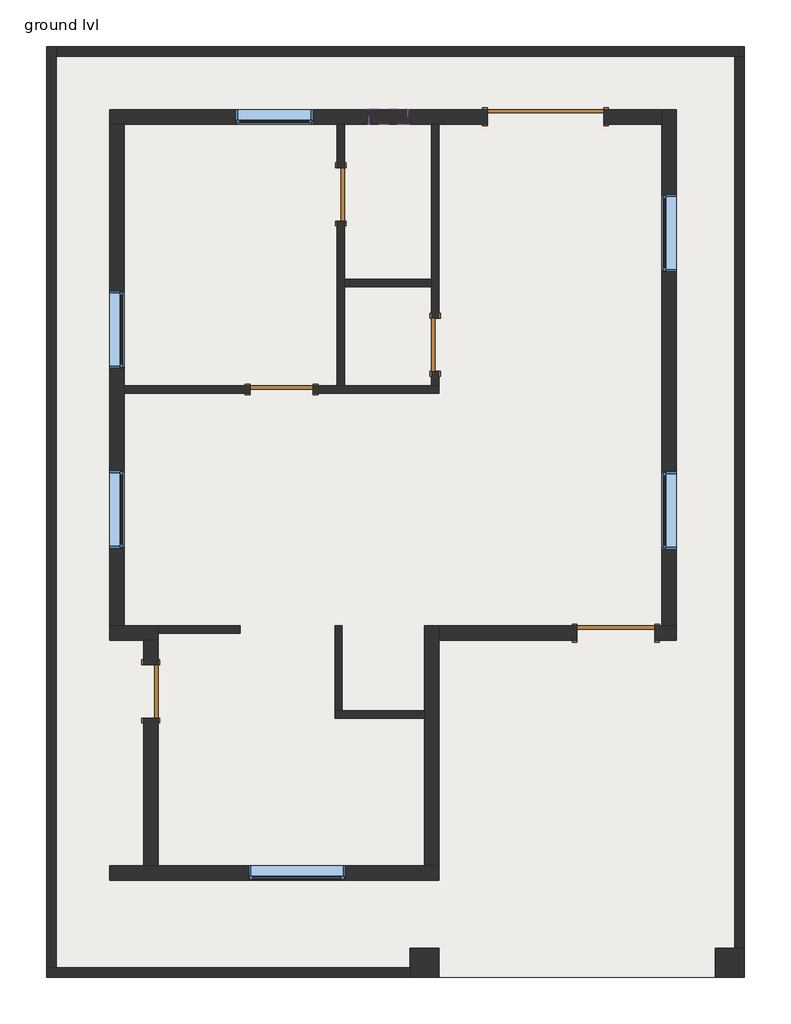
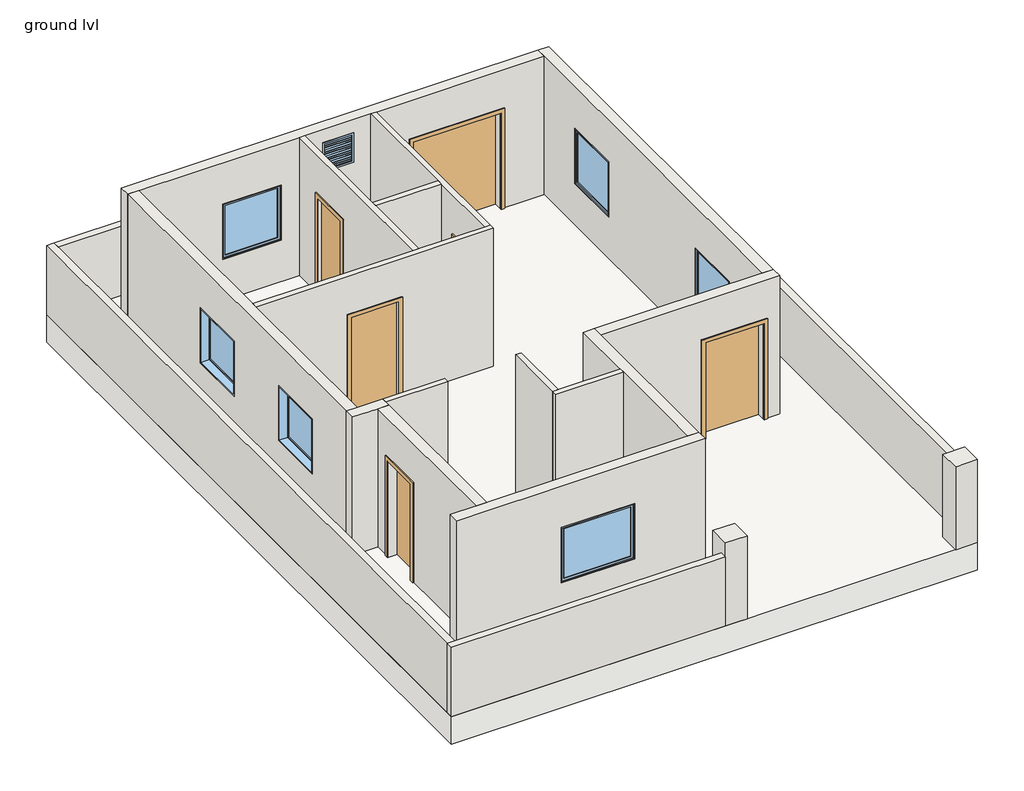
# One storey: 21 walls, 7 windows, 6 doors, 1 slab.
"""IFC4 building model written with IfcOpenShell, lengths in millimetres."""

from ifc_helpers import new_model, si_unit, frame, origin, origin_with_axes, place, context, project, spatial, polyline, outline, extrude, faceted_brep, transform, mapped, element, save
from components import single_flush_6_d_bd5e0b13, single_flush_d1_2531c3a3, single_flush_d2_53d9c022, single_flush_d3_0217d254, single_flush_d4_f1814d11, single_flush_d2_19300210, fixed_4_2_76f305d9, fixed_5_145d3b12, window_louvers_2_f2d8fef0

model = new_model("IFC4")

# Units and contexts
model_context = context("Model", 3, world=origin())
ifc_project = project(units=[si_unit("LENGTHUNIT", "METRE", prefix="MILLI")], contexts=[model_context])

# Site, building, storey
site = spatial("IfcSite", under=ifc_project)
building = spatial("IfcBuilding", under=site)
storey = spatial("IfcBuildingStorey", under=building, Name="ground lvl", Elevation=0.0)

# Doors
placement = place(None, origin())
single_flush_6_d_shape = single_flush_6_d_bd5e0b13(model_context)
element("IfcDoor", 1, ObjectType="Single-Flush : 6' d", at=placement, inside=storey, context=model_context, shape_type="MappedRepresentation", body=[
    mapped(single_flush_6_d_shape, transform((-16061.6899593, 8004.4908098, 0.0), x_axis=(1.0, 0.0, 0.0), y_axis=(0.0, 1.0, 0.0), z_axis=(0.0, 0.0, 1.0))),
])
single_flush_d1_shape = single_flush_d1_2531c3a3(model_context)
element("IfcDoor", 2, ObjectType="Single-Flush : d1", at=placement, inside=storey, context=model_context, shape_type="MappedRepresentation", body=[
    mapped(single_flush_d1_shape, transform((-14956.7899593, -110.8091902, 0.0), x_axis=(1.0, 0.0, 0.0), y_axis=(0.0, 1.0, 0.0), z_axis=(0.0, 0.0, 1.0))),
])
single_flush_d2_shape = single_flush_d2_53d9c022(model_context)
element("IfcDoor", 3, ObjectType="Single-Flush : d2", at=placement, inside=storey, context=model_context, shape_type="MappedRepresentation", body=[
    mapped(single_flush_d2_shape, transform((-22271.9899593, -1025.2091902, 0.0), x_axis=(0.0, 1.0, 0.0), y_axis=(-1.0, 0.0, 0.0), z_axis=(0.0, 0.0, 1.0))),
])
single_flush_d3_shape = single_flush_d3_0217d254(model_context)
element("IfcDoor", 4, ObjectType="Single-Flush : d3", at=placement, inside=storey, context=model_context, shape_type="MappedRepresentation", body=[
    mapped(single_flush_d3_shape, transform((-20214.5899593, 3718.2408098, 0.0), x_axis=(1.0, 0.0, 0.0), y_axis=(0.0, 1.0, 0.0), z_axis=(0.0, 0.0, 1.0))),
])
single_flush_d4_shape = single_flush_d4_f1814d11(model_context)
element("IfcDoor", 5, ObjectType="Single-Flush : d4", at=placement, inside=storey, context=model_context, shape_type="MappedRepresentation", body=[
    mapped(single_flush_d4_shape, transform((-19281.1399593, 6785.2908098, 0.0), x_axis=(0.0, -1.0, 0.0), y_axis=(1.0, 0.0, 0.0), z_axis=(0.0, 0.0, 1.0))),
])
single_flush_d2_2_shape = single_flush_d2_19300210(model_context)
element("IfcDoor", 6, ObjectType="Single-Flush : d4", at=placement, inside=storey, context=model_context, shape_type="MappedRepresentation", body=[
    mapped(single_flush_d2_2_shape, transform((-17795.2399593, 4423.0908098, 0.0), x_axis=(0.0, -1.0, 0.0), y_axis=(1.0, 0.0, 0.0), z_axis=(0.0, 0.0, 1.0))),
])

# Slab
element("IfcSlab", 7, ObjectType="2'", at=placement, inside=storey, context=model_context, shape_type="SweptSolid", body=[
    extrude(outline(polyline([(-23910.2899593, 9109.3908098), (-12937.4899593, 9109.3908098), (-12937.4899593, -5521.0091902), (-23910.2899593, -5521.0091902), (-23910.2899593, 9109.3908098)])), frame((0.0, 0.0, -609.6), z_axis=(0.0, 0.0, 1.0), x_axis=(1.0, 0.0, 0.0)), (0.0, 0.0, 1.0), 609.6),
])

# Walls
element("IfcWall", 8, ObjectType="1'6\" w", at=placement, inside=storey, context=model_context, shape_type="Brep", body=[
    faceted_brep([(-18195.2899593, -5521.0091902, 0.0), (-17738.0899593, -5521.0091902, 0.0), (-17738.0899593, -5521.0091902, 1828.8), (-18195.2899593, -5521.0091902, 1828.8), (-18195.2899593, -5521.0091902, 1524.0), (-18195.2899593, -5063.8091902, 0.0), (-18195.2899593, -5063.8091902, 1828.8), (-17738.0899593, -5063.8091902, 1828.8), (-17738.0899593, -5063.8091902, 0.0), (-18195.2899593, -5368.6091902, 0.0)], [[[0, 1, 2, 3, 4]], [[5, 6, 7, 8]], [[1, 0, 9, 5, 8]], [[2, 1, 8, 7]], [[3, 2, 7, 6]], [[0, 4, 3, 6, 5, 9]]]),
])
element("IfcWall", 9, ObjectType="1'6\" w", at=placement, inside=storey, context=model_context, shape_type="Brep", body=[
    faceted_brep([(-13394.6899593, -5521.0091902, 0.0), (-12937.4899593, -5521.0091902, 0.0), (-12937.4899593, -5521.0091902, 1828.8), (-13394.6899593, -5521.0091902, 1828.8), (-13394.6899593, -5063.8091902, 0.0), (-13394.6899593, -5063.8091902, 1828.8), (-12937.4899593, -5063.8091902, 1828.8), (-12937.4899593, -5063.8091902, 1524.0), (-12937.4899593, -5063.8091902, 0.0), (-13089.8899593, -5063.8091902, 0.0)], [[[0, 1, 2, 3]], [[4, 5, 6, 7, 8, 9]], [[1, 0, 4, 9, 8]], [[3, 2, 6, 5]], [[0, 3, 5, 4]], [[2, 1, 8, 7, 6]]]),
])
element("IfcWall", 10, ObjectType="4.5\" w", at=placement, inside=storey, context=model_context, shape_type="SweptSolid", body=[
    extrude(outline(polyline([(-20862.2899593, -110.8091902), (-22157.6899593, -110.8091902), (-22157.6899593, 3.4908098), (-20862.2899593, 3.4908098), (-20862.2899593, -110.8091902)])), origin_with_axes(), (0.0, 0.0, 1.0), 3048.0),
])
element("IfcWall", 11, ObjectType="4.5\" w", at=placement, inside=storey, context=model_context, shape_type="Brep", body=[
    faceted_brep([(-17966.6899593, -1330.0091901, 0.0), (-19262.0899593, -1330.0091901, 0.0), (-19376.3899593, -1330.0091901, 0.0), (-19376.3899593, -1330.0091901, 3048.0), (-19262.0899593, -1330.0091901, 3048.0), (-17966.6899593, -1330.0091901, 3048.0), (-17966.6899593, -1444.3091901, 0.0), (-17966.6899593, -1444.3091901, 3048.0), (-19376.3899593, -1444.3091901, 3048.0), (-19376.3899593, -1444.3091901, 0.0)], [[[0, 1, 2, 3, 4, 5]], [[6, 7, 8, 9]], [[2, 1, 0, 6, 9]], [[5, 4, 3, 8, 7]], [[0, 5, 7, 6]], [[3, 2, 9, 8]]]),
])
element("IfcWall", 12, ObjectType="4.5\" w", at=placement, inside=storey, context=model_context, shape_type="SweptSolid", body=[
    extrude(outline(polyline([(-19262.0899593, 3.4908098), (-19262.0899593, -1330.0091901), (-19376.3899593, -1330.0091901), (-19376.3899593, 3.4908098), (-19262.0899593, 3.4908098)])), origin_with_axes(), (0.0, 0.0, 1.0), 3048.0),
])
element("IfcWall", 13, ObjectType="4.5\" w", at=placement, inside=storey, context=model_context, shape_type="Brep", body=[
    faceted_brep([(-19719.2899593, 3661.0908098, 2133.6), (-19719.2899593, 3661.0908098, 0.0), (-17738.0899593, 3661.0908098, 0.0), (-17738.0899593, 3661.0908098, 3048.0), (-22691.0899593, 3661.0908098, 3048.0), (-22691.0899593, 3661.0908098, 0.0), (-20709.8899593, 3661.0908098, 0.0), (-20709.8899593, 3661.0908098, 2133.6), (-17738.0899593, 3775.3908098, 0.0), (-17852.3899593, 3775.3908098, 0.0), (-19223.9899593, 3775.3908098, 0.0), (-19338.2899593, 3775.3908098, 0.0), (-19719.2899593, 3775.3908098, 0.0), (-19719.2899593, 3775.3908098, 2133.6), (-20709.8899593, 3775.3908098, 2133.6), (-20709.8899593, 3775.3908098, 0.0), (-22691.0899593, 3775.3908098, 0.0), (-22691.0899593, 3775.3908098, 3048.0), (-19338.2899593, 3775.3908098, 3048.0), (-19223.9899593, 3775.3908098, 3048.0), (-17852.3899593, 3775.3908098, 3048.0), (-17738.0899593, 3775.3908098, 3048.0)], [[[0, 1, 2, 3, 4, 5, 6, 7]], [[8, 9, 10, 11, 12, 13, 14, 15, 16, 17, 18, 19, 20, 21]], [[6, 5, 16, 15]], [[2, 1, 12, 11, 10, 9, 8]], [[4, 3, 21, 20, 19, 18, 17]], [[5, 4, 17, 16]], [[3, 2, 8, 21]], [[13, 12, 1, 0]], [[14, 13, 0, 7]], [[15, 14, 7, 6]]]),
])
element("IfcWall", 14, ObjectType="4.5\" w", at=placement, inside=storey, context=model_context, shape_type="Brep", body=[
    faceted_brep([(-17738.0899593, 3775.3908098, 0.0), (-17738.0899593, 4003.9908098, 0.0), (-17738.0899593, 4003.9908098, 2133.6), (-17738.0899593, 4842.1908098, 2133.6), (-17738.0899593, 4842.1908098, 0.0), (-17738.0899593, 7890.1908098, 0.0), (-17738.0899593, 7890.1908098, 3048.0), (-17738.0899593, 3775.3908098, 3048.0), (-17852.3899593, 4003.9908098, 2133.6), (-17852.3899593, 4003.9908098, 0.0), (-17852.3899593, 3775.3908098, 0.0), (-17852.3899593, 3775.3908098, 3048.0), (-17852.3899593, 5337.4908098, 3048.0), (-17852.3899593, 5451.7908098, 3048.0), (-17852.3899593, 7890.1908098, 3048.0), (-17852.3899593, 7890.1908098, 0.0), (-17852.3899593, 5451.7908098, 0.0), (-17852.3899593, 5337.4908098, 0.0), (-17852.3899593, 4842.1908098, 0.0), (-17852.3899593, 4842.1908098, 2133.6)], [[[0, 1, 2, 3, 4, 5, 6, 7]], [[8, 9, 10, 11, 12, 13, 14, 15, 16, 17, 18, 19]], [[10, 9, 1, 0]], [[18, 17, 16, 15, 5, 4]], [[7, 6, 14, 13, 12, 11]], [[0, 7, 11, 10]], [[6, 5, 15, 14]], [[2, 1, 9, 8]], [[3, 2, 8, 19]], [[4, 3, 19, 18]]]),
])
element("IfcWall", 15, ObjectType="4.5\" w", at=placement, inside=storey, context=model_context, shape_type="Brep", body=[
    faceted_brep([(-19223.9899593, 3775.3908098, 0.0), (-19223.9899593, 5337.4908098, 0.0), (-19223.9899593, 5451.7908098, 0.0), (-19223.9899593, 6366.1908098, 0.0), (-19223.9899593, 6366.1908098, 2133.6), (-19223.9899593, 7204.3908098, 2133.6), (-19223.9899593, 7204.3908098, 0.0), (-19223.9899593, 7890.1908098, 0.0), (-19223.9899593, 7890.1908098, 3048.0), (-19223.9899593, 5451.7908098, 3048.0), (-19223.9899593, 5337.4908098, 3048.0), (-19223.9899593, 3775.3908098, 3048.0), (-19338.2899593, 6366.1908098, 2133.6), (-19338.2899593, 6366.1908098, 0.0), (-19338.2899593, 3775.3908098, 0.0), (-19338.2899593, 3775.3908098, 3048.0), (-19338.2899593, 7890.1908098, 3048.0), (-19338.2899593, 7890.1908098, 0.0), (-19338.2899593, 7204.3908098, 0.0), (-19338.2899593, 7204.3908098, 2133.6)], [[[0, 1, 2, 3, 4, 5, 6, 7, 8, 9, 10, 11]], [[12, 13, 14, 15, 16, 17, 18, 19]], [[18, 17, 7, 6]], [[14, 13, 3, 2, 1, 0]], [[11, 10, 9, 8, 16, 15]], [[8, 7, 17, 16]], [[0, 11, 15, 14]], [[4, 3, 13, 12]], [[5, 4, 12, 19]], [[6, 5, 19, 18]]]),
])
element("IfcWall", 16, ObjectType="4.5\" w", at=placement, inside=storey, context=model_context, shape_type="SweptSolid", body=[
    extrude(outline(polyline([(-17852.3899593, 5337.4908098), (-19223.9899593, 5337.4908098), (-19223.9899593, 5451.7908098), (-17852.3899593, 5451.7908098), (-17852.3899593, 5337.4908098)])), origin_with_axes(), (0.0, 0.0, 1.0), 3048.0),
])
element("IfcWall", 17, ObjectType="6\" w", at=placement, inside=storey, context=model_context, shape_type="Brep", body=[
    faceted_brep([(-18195.2899593, -5368.6091902, 0.0), (-23757.8899593, -5368.6091902, 0.0), (-23910.2899593, -5368.6091902, 0.0), (-23910.2899593, -5368.6091902, 1524.0), (-23757.8899593, -5368.6091902, 1524.0), (-18195.2899593, -5368.6091902, 1524.0), (-18195.2899593, -5521.0091902, 0.0), (-18195.2899593, -5521.0091902, 1524.0), (-23910.2899593, -5521.0091902, 1524.0), (-23910.2899593, -5521.0091902, 0.0)], [[[0, 1, 2, 3, 4, 5]], [[6, 7, 8, 9]], [[2, 1, 0, 6, 9]], [[5, 4, 3, 8, 7]], [[0, 5, 7, 6]], [[3, 2, 9, 8]]]),
])
element("IfcWall", 18, ObjectType="6\" w", at=placement, inside=storey, context=model_context, shape_type="Brep", body=[
    faceted_brep([(-23757.8899593, -5368.6091902, 0.0), (-23757.8899593, 8956.9908098, 0.0), (-23757.8899593, 9109.3908098, 0.0), (-23757.8899593, 9109.3908098, 1524.0), (-23757.8899593, 8956.9908098, 1524.0), (-23757.8899593, -5368.6091902, 1524.0), (-23910.2899593, -5368.6091902, 0.0), (-23910.2899593, -5368.6091902, 1524.0), (-23910.2899593, 9109.3908098, 1524.0), (-23910.2899593, 9109.3908098, 0.0)], [[[0, 1, 2, 3, 4, 5]], [[6, 7, 8, 9]], [[2, 1, 0, 6, 9]], [[5, 4, 3, 8, 7]], [[0, 5, 7, 6]], [[3, 2, 9, 8]]]),
])
element("IfcWall", 19, ObjectType="6\" w", at=placement, inside=storey, context=model_context, shape_type="Brep", body=[
    faceted_brep([(-23757.8899593, 8956.9908098, 0.0), (-13089.8899593, 8956.9908098, 0.0), (-12937.4899593, 8956.9908098, 0.0), (-12937.4899593, 8956.9908098, 1524.0), (-13089.8899593, 8956.9908098, 1524.0), (-23757.8899593, 8956.9908098, 1524.0), (-23757.8899593, 9109.3908098, 0.0), (-23757.8899593, 9109.3908098, 1524.0), (-12937.4899593, 9109.3908098, 1524.0), (-12937.4899593, 9109.3908098, 0.0)], [[[0, 1, 2, 3, 4, 5]], [[6, 7, 8, 9]], [[2, 1, 0, 6, 9]], [[5, 4, 3, 8, 7]], [[0, 5, 7, 6]], [[3, 2, 9, 8]]]),
])
element("IfcWall", 20, ObjectType="6\" w", at=placement, inside=storey, context=model_context, shape_type="SweptSolid", body=[
    extrude(outline(polyline([(-13089.8899593, -5063.8091902), (-13089.8899593, 8956.9908098), (-12937.4899593, 8956.9908098), (-12937.4899593, -5063.8091902), (-13089.8899593, -5063.8091902)])), origin_with_axes(), (0.0, 0.0, 1.0), 1524.0),
])
element("IfcWall", 21, ObjectType="9\" w", at=placement, inside=storey, context=model_context, shape_type="Brep", body=[
    faceted_brep([(-22919.6899593, -3997.0091902, 0.0), (-17738.0899593, -3997.0091902, 0.0), (-17738.0899593, -3997.0091902, 3048.0), (-22919.6899593, -3997.0091902, 3048.0), (-20735.2080965, -3997.0091902, 2133.6), (-19211.2080965, -3997.0091902, 2133.6), (-19211.2080965, -3997.0091902, 914.4), (-20735.2080965, -3997.0091902, 914.4), (-22919.6899593, -3768.4091902, 0.0), (-22919.6899593, -3768.4091902, 3048.0), (-22386.2899593, -3768.4091902, 3048.0), (-22157.6899593, -3768.4091902, 3048.0), (-17966.6899593, -3768.4091902, 3048.0), (-17738.0899593, -3768.4091902, 3048.0), (-17738.0899593, -3768.4091902, 0.0), (-17966.6899593, -3768.4091902, 0.0), (-22157.6899593, -3768.4091902, 0.0), (-22386.2899593, -3768.4091902, 0.0), (-20735.2080965, -3768.4091902, 2133.6), (-20735.2080965, -3768.4091902, 914.4), (-19211.2080965, -3768.4091902, 914.4), (-19211.2080965, -3768.4091902, 2133.6)], [[[0, 1, 2, 3], [4, 5, 6, 7]], [[8, 9, 10, 11, 12, 13, 14, 15, 16, 17], [18, 19, 20, 21]], [[1, 0, 8, 17, 16, 15, 14]], [[3, 2, 13, 12, 11, 10, 9]], [[0, 3, 9, 8]], [[2, 1, 14, 13]], [[19, 18, 4, 7]], [[20, 19, 7, 6]], [[21, 20, 6, 5]], [[18, 21, 5, 4]]]),
])
element("IfcWall", 22, ObjectType="9\" w", at=placement, inside=storey, context=model_context, shape_type="Brep", body=[
    faceted_brep([(-17738.0899593, -3768.4091902, 0.0), (-17738.0899593, -225.1091902, 0.0), (-17738.0899593, 3.4908098, 0.0), (-17738.0899593, 3.4908098, 3048.0), (-17738.0899593, -225.1091902, 3048.0), (-17738.0899593, -3768.4091902, 3048.0), (-17966.6899593, -3768.4091902, 0.0), (-17966.6899593, -3768.4091902, 3048.0), (-17966.6899593, -1444.3091901, 3048.0), (-17966.6899593, -1330.0091901, 3048.0), (-17966.6899593, 3.4908098, 3048.0), (-17966.6899593, 3.4908098, 0.0), (-17966.6899593, -1330.0091901, 0.0), (-17966.6899593, -1444.3091901, 0.0)], [[[0, 1, 2, 3, 4, 5]], [[6, 7, 8, 9, 10, 11, 12, 13]], [[2, 1, 0, 6, 13, 12, 11]], [[5, 4, 3, 10, 9, 8, 7]], [[0, 5, 7, 6]], [[3, 2, 11, 10]]]),
])
element("IfcWall", 23, ObjectType="9\" w", at=placement, inside=storey, context=model_context, shape_type="Brep", body=[
    faceted_brep([(-14347.1899593, -225.1091902, 2133.6), (-14347.1899593, -225.1091902, 0.0), (-14004.2899593, -225.1091902, 0.0), (-14004.2899593, -225.1091902, 3048.0), (-17738.0899593, -225.1091902, 3048.0), (-17738.0899593, -225.1091902, 0.0), (-15566.3899593, -225.1091902, 0.0), (-15566.3899593, -225.1091902, 2133.6), (-14004.2899593, 3.4908098, 0.0), (-14232.8899593, 3.4908098, 0.0), (-14347.1899593, 3.4908098, 0.0), (-14347.1899593, 3.4908098, 2133.6), (-15566.3899593, 3.4908098, 2133.6), (-15566.3899593, 3.4908098, 0.0), (-17738.0899593, 3.4908098, 0.0), (-17738.0899593, 3.4908098, 3048.0), (-14232.8899593, 3.4908098, 3048.0), (-14004.2899593, 3.4908098, 3048.0)], [[[0, 1, 2, 3, 4, 5, 6, 7]], [[8, 9, 10, 11, 12, 13, 14, 15, 16, 17]], [[6, 5, 14, 13]], [[2, 1, 10, 9, 8]], [[4, 3, 17, 16, 15]], [[5, 4, 15, 14]], [[3, 2, 8, 17]], [[11, 10, 1, 0]], [[12, 11, 0, 7]], [[13, 12, 7, 6]]]),
])
element("IfcWall", 24, ObjectType="9\" w", at=placement, inside=storey, context=model_context, shape_type="Brep", body=[
    faceted_brep([(-14004.2899593, 3.4908098, 0.0), (-14004.2899593, 8118.7908098, 0.0), (-14004.2899593, 8118.7908098, 3048.0), (-14004.2899593, 3.4908098, 3048.0), (-14004.2899593, 2429.1908098, 2133.6), (-14004.2899593, 2429.1908098, 914.4), (-14004.2899593, 1209.9908098, 914.4), (-14004.2899593, 1209.9908098, 2133.6), (-14004.2899593, 6785.2908098, 2133.6), (-14004.2899593, 6785.2908098, 914.4), (-14004.2899593, 5566.0908098, 914.4), (-14004.2899593, 5566.0908098, 2133.6), (-14232.8899593, 3.4908098, 0.0), (-14232.8899593, 3.4908098, 3048.0), (-14232.8899593, 7890.1908098, 3048.0), (-14232.8899593, 8118.7908098, 3048.0), (-14232.8899593, 8118.7908098, 0.0), (-14232.8899593, 7890.1908098, 0.0), (-14232.8899593, 2429.1908098, 2133.6), (-14232.8899593, 1209.9908098, 2133.6), (-14232.8899593, 1209.9908098, 914.4), (-14232.8899593, 2429.1908098, 914.4), (-14232.8899593, 6785.2908098, 2133.6), (-14232.8899593, 5566.0908098, 2133.6), (-14232.8899593, 5566.0908098, 914.4), (-14232.8899593, 6785.2908098, 914.4)], [[[0, 1, 2, 3], [4, 5, 6, 7], [8, 9, 10, 11]], [[12, 13, 14, 15, 16, 17], [18, 19, 20, 21], [22, 23, 24, 25]], [[1, 0, 12, 17, 16]], [[3, 2, 15, 14, 13]], [[0, 3, 13, 12]], [[2, 1, 16, 15]], [[5, 4, 18, 21]], [[6, 5, 21, 20]], [[7, 6, 20, 19]], [[4, 7, 19, 18]], [[9, 8, 22, 25]], [[10, 9, 25, 24]], [[11, 10, 24, 23]], [[8, 11, 23, 22]]]),
])
element("IfcWall", 25, ObjectType="9\" w", at=placement, inside=storey, context=model_context, shape_type="Brep", body=[
    faceted_brep([(-14232.8899593, 8118.7908098, 0.0), (-15147.2899593, 8118.7908098, 0.0), (-15147.2899593, 8118.7908098, 2133.6), (-16976.0899593, 8118.7908098, 2133.6), (-16976.0899593, 8118.7908098, 0.0), (-22919.6899593, 8118.7908098, 0.0), (-22919.6899593, 8118.7908098, 3048.0), (-14232.8899593, 8118.7908098, 3048.0), (-20938.4899593, 8118.7908098, 2133.6), (-20938.4899593, 8118.7908098, 914.4), (-19719.2899593, 8118.7908098, 914.4), (-19719.2899593, 8118.7908098, 2133.6), (-18230.9643658, 8118.7908098, 2743.2), (-18840.5643658, 8118.7908098, 2743.2), (-18840.5643658, 8118.7908098, 2133.6), (-18230.9643658, 8118.7908098, 2133.6), (-15147.2899593, 7890.1908098, 2133.6), (-15147.2899593, 7890.1908098, 0.0), (-14232.8899593, 7890.1908098, 0.0), (-14232.8899593, 7890.1908098, 3048.0), (-17738.0899593, 7890.1908098, 3048.0), (-17852.3899593, 7890.1908098, 3048.0), (-19223.9899593, 7890.1908098, 3048.0), (-19338.2899593, 7890.1908098, 3048.0), (-22691.0899593, 7890.1908098, 3048.0), (-22919.6899593, 7890.1908098, 3048.0), (-22919.6899593, 7890.1908098, 0.0), (-22691.0899593, 7890.1908098, 0.0), (-19338.2899593, 7890.1908098, 0.0), (-19223.9899593, 7890.1908098, 0.0), (-17852.3899593, 7890.1908098, 0.0), (-17738.0899593, 7890.1908098, 0.0), (-16976.0899593, 7890.1908098, 0.0), (-16976.0899593, 7890.1908098, 2133.6), (-20938.4899593, 7890.1908098, 2133.6), (-19719.2899593, 7890.1908098, 2133.6), (-19719.2899593, 7890.1908098, 914.4), (-20938.4899593, 7890.1908098, 914.4), (-18230.9643658, 7890.1908098, 2743.2), (-18230.9643658, 7890.1908098, 2133.6), (-18840.5643658, 7890.1908098, 2133.6), (-18840.5643658, 7890.1908098, 2743.2)], [[[0, 1, 2, 3, 4, 5, 6, 7], [8, 9, 10, 11], [12, 13, 14, 15]], [[16, 17, 18, 19, 20, 21, 22, 23, 24, 25, 26, 27, 28, 29, 30, 31, 32, 33], [34, 35, 36, 37], [38, 39, 40, 41]], [[18, 17, 1, 0]], [[32, 31, 30, 29, 28, 27, 26, 5, 4]], [[7, 6, 25, 24, 23, 22, 21, 20, 19]], [[0, 7, 19, 18]], [[6, 5, 26, 25]], [[9, 8, 34, 37]], [[10, 9, 37, 36]], [[11, 10, 36, 35]], [[8, 11, 35, 34]], [[39, 38, 12, 15]], [[40, 39, 15, 14]], [[41, 40, 14, 13]], [[38, 41, 13, 12]], [[2, 1, 17, 16]], [[3, 2, 16, 33]], [[4, 3, 33, 32]]]),
])
element("IfcWall", 26, ObjectType="9\" w", at=placement, inside=storey, context=model_context, shape_type="Brep", body=[
    faceted_brep([(-22919.6899593, 7890.1908098, 0.0), (-22919.6899593, 3.4908098, 0.0), (-22919.6899593, 3.4908098, 3048.0), (-22919.6899593, 7890.1908098, 3048.0), (-22919.6899593, 4050.7074782, 2133.6), (-22919.6899593, 4050.7074782, 914.4), (-22919.6899593, 5269.9074782, 914.4), (-22919.6899593, 5269.9074782, 2133.6), (-22919.6899593, 1222.6908095, 2133.6), (-22919.6899593, 1222.6908095, 914.4), (-22919.6899593, 2441.8908095, 914.4), (-22919.6899593, 2441.8908095, 2133.6), (-22691.0899593, 7890.1908098, 0.0), (-22691.0899593, 7890.1908098, 3048.0), (-22691.0899593, 3775.3908098, 3048.0), (-22691.0899593, 3661.0908098, 3048.0), (-22691.0899593, 3.4908098, 3048.0), (-22691.0899593, 3.4908098, 0.0), (-22691.0899593, 3661.0908098, 0.0), (-22691.0899593, 3775.3908098, 0.0), (-22691.0899593, 4050.7074782, 2133.6), (-22691.0899593, 5269.9074782, 2133.6), (-22691.0899593, 5269.9074782, 914.4), (-22691.0899593, 4050.7074782, 914.4), (-22691.0899593, 1222.6908095, 2133.6), (-22691.0899593, 2441.8908095, 2133.6), (-22691.0899593, 2441.8908095, 914.4), (-22691.0899593, 1222.6908095, 914.4)], [[[0, 1, 2, 3], [4, 5, 6, 7], [8, 9, 10, 11]], [[12, 13, 14, 15, 16, 17, 18, 19], [20, 21, 22, 23], [24, 25, 26, 27]], [[1, 0, 12, 19, 18, 17]], [[3, 2, 16, 15, 14, 13]], [[0, 3, 13, 12]], [[2, 1, 17, 16]], [[5, 4, 20, 23]], [[6, 5, 23, 22]], [[7, 6, 22, 21]], [[4, 7, 21, 20]], [[9, 8, 24, 27]], [[10, 9, 27, 26]], [[11, 10, 26, 25]], [[8, 11, 25, 24]]]),
])
element("IfcWall", 27, ObjectType="9\" w", at=placement, inside=storey, context=model_context, shape_type="Brep", body=[
    faceted_brep([(-22919.6899593, -225.1091902, 0.0), (-22386.2899593, -225.1091902, 0.0), (-22157.6899593, -225.1091902, 0.0), (-22157.6899593, -225.1091902, 3048.0), (-22386.2899593, -225.1091902, 3048.0), (-22919.6899593, -225.1091902, 3048.0), (-22919.6899593, 3.4908098, 0.0), (-22919.6899593, 3.4908098, 3048.0), (-22691.0899593, 3.4908098, 3048.0), (-22157.6899593, 3.4908098, 3048.0), (-22157.6899593, 3.4908098, 0.0), (-22691.0899593, 3.4908098, 0.0), (-22157.6899593, -110.8091902, 0.0), (-22157.6899593, -110.8091902, 3048.0)], [[[0, 1, 2, 3, 4, 5]], [[6, 7, 8, 9, 10, 11]], [[2, 1, 0, 6, 11, 10, 12]], [[5, 4, 3, 13, 9, 8, 7]], [[0, 5, 7, 6]], [[3, 2, 12, 10, 9, 13]]]),
])
element("IfcWall", 28, ObjectType="9\" w", at=placement, inside=storey, context=model_context, shape_type="SweptSolid", body=[
    extrude(outline(polyline([(-225.1091902, 0.0), (-606.1091902, 0.0), (-606.1091902, 2133.6), (-1444.3091902, 2133.6), (-1444.3091902, 0.0), (-3768.4091902, 0.0), (-3768.4091902, 3048.0), (-225.1091902, 3048.0), (-225.1091902, 0.0)])), frame((-22386.2899593, 0.0, 0.0), z_axis=(1.0, 0.0, 0.0), x_axis=(0.0, 1.0, 0.0)), (0.0, 0.0, 1.0), 228.6),
])

# Windows
fixed_4_2_shape = fixed_4_2_76f305d9(model_context)
element("IfcWindow", 29, ObjectType="Fixed : 4'", at=placement, inside=storey, context=model_context, shape_type="MappedRepresentation", body=[
    mapped(fixed_4_2_shape, transform((-14118.5899593, 6213.7908098, 0.0), x_axis=(0.0, 1.0, 0.0), y_axis=(-1.0, 0.0, 0.0), z_axis=(0.0, 0.0, 1.0))),
])
element("IfcWindow", 30, ObjectType="Fixed : 4'", at=placement, inside=storey, context=model_context, shape_type="MappedRepresentation", body=[
    mapped(fixed_4_2_shape, transform((-20366.9899593, 8004.4908098, 0.0), x_axis=(-1.0, 0.0, 0.0), y_axis=(0.0, -1.0, 0.0), z_axis=(0.0, 0.0, 1.0))),
])
element("IfcWindow", 31, ObjectType="Fixed : 4'", at=placement, inside=storey, context=model_context, shape_type="MappedRepresentation", body=[
    mapped(fixed_4_2_shape, transform((-22805.3899593, 4622.2074782, 0.0), x_axis=(0.0, -1.0, 0.0), y_axis=(1.0, 0.0, 0.0), z_axis=(0.0, 0.0, 1.0))),
])
element("IfcWindow", 32, ObjectType="Fixed : 4'", at=placement, inside=storey, context=model_context, shape_type="MappedRepresentation", body=[
    mapped(fixed_4_2_shape, transform((-22805.3899593, 1794.1908095, 0.0), x_axis=(0.0, -1.0, 0.0), y_axis=(1.0, 0.0, 0.0), z_axis=(0.0, 0.0, 1.0))),
])
element("IfcWindow", 33, ObjectType="Fixed : 4' 2", at=placement, inside=storey, context=model_context, shape_type="MappedRepresentation", body=[
    mapped(fixed_4_2_shape, transform((-14118.5899593, 1857.6908098, 0.0), x_axis=(0.0, 1.0, 0.0), y_axis=(-1.0, 0.0, 0.0), z_axis=(0.0, 0.0, 1.0))),
])
fixed_5_shape = fixed_5_145d3b12(model_context)
element("IfcWindow", 34, ObjectType="Fixed : 5'", at=placement, inside=storey, context=model_context, shape_type="MappedRepresentation", body=[
    mapped(fixed_5_shape, transform((-20011.3080965, -3882.7091902, 0.0), x_axis=(-1.0, 0.0, 0.0), y_axis=(0.0, -1.0, 0.0), z_axis=(0.0, 0.0, 1.0))),
])
window_louvers_2_shape = window_louvers_2_f2d8fef0(model_context)
element("IfcWindow", 35, ObjectType="Window-Louvers : 24\" x 24\"", at=placement, inside=storey, context=model_context, shape_type="MappedRepresentation", body=[
    mapped(window_louvers_2_shape, transform((-18535.7643658, 7998.1408098, 1219.2), x_axis=(-1.0, 0.0, 0.0), y_axis=(0.0, -1.0, 0.0), z_axis=(0.0, 0.0, 1.0))),
])

save(model, "model.ifc")

# Revit data of these elements
# Type "Single-Flush : 6' d"
#   Type Mark = "12"
#   Construction Type Id = "MDOOR"
#   Assembly Code = "C1020"
#   Analytic Construction = "Metal"
#   Thickness = 0' - 2"
#   Heat Transfer Coefficient (U) = 0.651978 BTU/(h·ft²·°F)
#   Height = 7' - 0"
#   Trim Projection Ext = 0' - 1"
#   Trim Projection Int = 0' - 1"
#   Trim Width = 0' - 3"
#   Width = 6' - 0"
#   Define Thermal Properties by = 1
#   Door Material = Door - Panel
#   Frame Material = Door - Frame
#   Visual Light Transmittance = 0
#   Solar Heat Gain Coefficient = 0
#   Function = (empty or 0)
#   Wall Closure = (empty or 0)
# Type "Single-Flush : d1"
#   Type Mark = "8"
#   Construction Type Id = "MDOOR"
#   Assembly Code = "C1020"
#   Analytic Construction = "Metal"
#   Thickness = 0' - 2"
#   Heat Transfer Coefficient (U) = 0.651978 BTU/(h·ft²·°F)
#   Height = 7' - 0"
#   Trim Projection Ext = 0' - 1"
#   Trim Projection Int = 0' - 1"
#   Trim Width = 0' - 3"
#   Width = 4' - 0"
#   Define Thermal Properties by = 1
#   Door Material = Door - Panel
#   Frame Material = Door - Frame
#   Visual Light Transmittance = 0
#   Solar Heat Gain Coefficient = 0
#   Function = (empty or 0)
#   Wall Closure = (empty or 0)
# Type "Single-Flush : d2"
#   Type Mark = "9"
#   Construction Type Id = "MDOOR"
#   Assembly Code = "C1020"
#   Analytic Construction = "Metal"
#   Thickness = 0' - 2"
#   Heat Transfer Coefficient (U) = 0.651978 BTU/(h·ft²·°F)
#   Height = 7' - 0"
#   Trim Projection Ext = 0' - 1"
#   Trim Projection Int = 0' - 1"
#   Trim Width = 0' - 3"
#   Width = 2' - 9"
#   Define Thermal Properties by = 1
#   Door Material = Door - Panel
#   Frame Material = Door - Frame
#   Visual Light Transmittance = 0
#   Solar Heat Gain Coefficient = 0
#   Function = (empty or 0)
#   Wall Closure = (empty or 0)
# Type "Single-Flush : d3"
#   Type Mark = "10"
#   Construction Type Id = "MDOOR"
#   Assembly Code = "C1020"
#   Analytic Construction = "Metal"
#   Thickness = 0' - 2"
#   Heat Transfer Coefficient (U) = 0.651978 BTU/(h·ft²·°F)
#   Height = 7' - 0"
#   Trim Projection Ext = 0' - 1"
#   Trim Projection Int = 0' - 1"
#   Trim Width = 0' - 3"
#   Width = 3' - 3"
#   Define Thermal Properties by = 1
#   Door Material = Door - Panel
#   Frame Material = Door - Frame
#   Visual Light Transmittance = 0
#   Solar Heat Gain Coefficient = 0
#   Function = (empty or 0)
#   Wall Closure = (empty or 0)
# Type "Single-Flush : d4"
#   Type Mark = "11"
#   Construction Type Id = "MDOOR"
#   Assembly Code = "C1020"
#   Analytic Construction = "Metal"
#   Thickness = 0' - 2"
#   Heat Transfer Coefficient (U) = 0.651978 BTU/(h·ft²·°F)
#   Height = 7' - 0"
#   Trim Projection Ext = 0' - 1"
#   Trim Projection Int = 0' - 1"
#   Trim Width = 0' - 3"
#   Width = 2' - 9"
#   Define Thermal Properties by = 1
#   Door Material = Door - Panel
#   Frame Material = Door - Frame
#   Visual Light Transmittance = 0
#   Solar Heat Gain Coefficient = 0
#   Function = (empty or 0)
#   Wall Closure = (empty or 0)
# Type "2'"
#   Assembly Code = "B1010"
#   Function = 0
#   Layers, outside or top first: 2' - 0" no material (function 1)
# Type "1'6\" w"
#   Assembly Code = "B2010"
#   Layers, outside or top first: 1' - 6" no material (function 1)
# Type "4.5\" w"
#   Assembly Code = "B2010"
#   Layers, outside or top first: 0' - 4 1/2" no material (function 1)
# Type "6\" w"
#   Assembly Code = "B2010"
#   Layers, outside or top first: 0' - 6" no material (function 1)
# Type "9\" w"
#   Assembly Code = "B2010"
#   Layers, outside or top first: 0' - 9" no material (function 1)
# Type "Fixed : 4'"
#   Type Mark = "19"
#   Construction Type Id = "GSP4R"
#   Assembly Code = "B2020100"
#   Analytic Construction = "1/8 in Pilkington single glazing"
#   Visual Light Transmittance = 0.9
#   Solar Heat Gain Coefficient = 0.78
#   Heat Transfer Coefficient (U) = 0.6496 BTU/(h·ft²·°F)
#   Height = 4' - 0"
#   Default Sill Height = 3' - 0"
#   Width = 4' - 0"
#   Window Inset = 0' - 0 3/4"
#   Define Thermal Properties by = 1
#   Glass Pane Material = Glass
#   Sash Material = Sash
#   Wall Closure = (empty or 0)
# Type "Fixed : 4' 2"
#   Type Mark = "20"
#   Construction Type Id = "GSP4R"
#   Assembly Code = "B2020100"
#   Analytic Construction = "1/8 in Pilkington single glazing"
#   Visual Light Transmittance = 0.9
#   Solar Heat Gain Coefficient = 0.78
#   Heat Transfer Coefficient (U) = 0.6496 BTU/(h·ft²·°F)
#   Height = 4' - 0"
#   Default Sill Height = 3' - 0"
#   Width = 4' - 0"
#   Window Inset = 0' - 0 3/4"
#   Define Thermal Properties by = 1
#   Glass Pane Material = Glass
#   Sash Material = Sash
#   Wall Closure = (empty or 0)
# Type "Fixed : 5'"
#   Type Mark = "18"
#   Construction Type Id = "GSP4R"
#   Assembly Code = "B2020100"
#   Analytic Construction = "1/8 in Pilkington single glazing"
#   Visual Light Transmittance = 0.9
#   Solar Heat Gain Coefficient = 0.78
#   Heat Transfer Coefficient (U) = 0.6496 BTU/(h·ft²·°F)
#   Height = 4' - 0"
#   Default Sill Height = 3' - 0"
#   Width = 5' - 0"
#   Window Inset = 0' - 0 3/4"
#   Define Thermal Properties by = 1
#   Glass Pane Material = Glass
#   Sash Material = Sash
#   Wall Closure = (empty or 0)
# Type "Window-Louvers : 24\" x 24\""
#   Type Mark = "21"
#   Construction Type Id = "GSP4R"
#   Assembly Code = "B20"
#   Analytic Construction = "1/8 in Pilkington single glazing"
#   Visual Light Transmittance = 0.9
#   Thermal Resistance (R) = 1.53941 (h·ft²·°F)/BTU
#   Solar Heat Gain Coefficient = 0.78
#   Max Height = 1' - 11.74264"
#   Height = 2' - 0"
#   Heat Transfer Coefficient (U) = 0.6496 BTU/(h·ft²·°F)
#   Blade Width [instance default] = 1' - 10 1/2"
#   Blade Vertical Thickness = 0' - 0.35355"
#   Blade Thickness = 0' - 0 1/4"
#   Blade Spacing = 0' - 1 1/2"
#   Blade Height = 0' - 1.85355"
#   Blade Depth = 0' - 3"
#   Blade Angle = 45.00°
#   Default Sill Height = 3' - 0"
#   Trim Projection_Exterior = 0' - 0 1/2"
#   Trim Projection_Interior = 0' - 0 1/2"
#   Trim Width_Exterior = 0' - 1 1/2"
#   Trim Width_Interior = 0' - 1 1/2"
#   Width = 2' - 0"
#   Max Blade Count = 12
#   Define Thermal Properties by = 1
#   Blade Count = 12
#   Frame Material = Birch
#   Louver Material = Birch
#   Trim Exterior Material = Birch
#   Trim Interior Material = Birch
#   Wall Closure = (empty or 0)
# Element 1 (IfcDoor, "Single-Flush : 6' d")
#   Phase Created = New Construction
#   Materials on its faces: "Door - Frame", "Door - Panel"
# Element 2 (IfcDoor, "Single-Flush : d1")
#   Phase Created = New Construction
#   Materials on its faces: "Door - Frame", "Door - Panel"
# Element 3 (IfcDoor, "Single-Flush : d2")
#   Phase Created = New Construction
#   Materials on its faces: "Door - Frame", "Door - Panel"
# Element 4 (IfcDoor, "Single-Flush : d3")
#   Phase Created = New Construction
#   Materials on its faces: "Door - Frame", "Door - Panel"
# Elements 5, 6 (IfcDoor, "Single-Flush : d4")
#   Phase Created = New Construction
#   Materials on its faces: "Door - Frame", "Door - Panel"
# Element 7 (IfcSlab, "2'")
#   built-in parameter 1001955 = 3.14159 (stored number, unit not read)
#   Height Offset From Level = 0' - 0"
#   Phase Created = New Construction
#   Materials on its faces: "Default Floor"
# Elements 8, 9 (IfcWall, "1'6\" w")
#   Top Offset = 0' - 0"
#   Base Offset = 0' - 0"
#   Unconnected Height = 6' - 0"
#   wall height = 6' - 0"
#   Phase Created = New Construction
#   Base Constraint = ground lvl
#   Materials on its faces: "Default Wall"
# Elements 10, 11, 12, 13, 14, 15, 16 (IfcWall, "4.5\" w")
#   Top Offset = 0' - 0"
#   Base Offset = 0' - 0"
#   Unconnected Height = 10' - 0"
#   wall height = 10' - 0"
#   Phase Created = New Construction
#   Base Constraint = ground lvl
#   Materials on its faces: "Default Wall"
# Elements 17, 18, 19, 20 (IfcWall, "6\" w")
#   Top Offset = 0' - 0"
#   Base Offset = 0' - 0"
#   Unconnected Height = 5' - 0"
#   wall height = 5' - 0"
#   Phase Created = New Construction
#   Base Constraint = ground lvl
#   Materials on its faces: "Default Wall"
# Elements 21, 22, 23, 24, 25, 26, 27, 28 (IfcWall, "9\" w")
#   Top Offset = 0' - 0"
#   Base Offset = 0' - 0"
#   Unconnected Height = 10' - 0"
#   wall height = 10' - 0"
#   Phase Created = New Construction
#   Base Constraint = ground lvl
#   Materials on its faces: "Default Wall"
# Element 29 (IfcWindow, "Fixed : 4'")
#   Mark = "3"
#   Phase Created = New Construction
#   Materials on its faces: "Sash", "Glass"
# Element 30 (IfcWindow, "Fixed : 4'")
#   Mark = "4"
#   Phase Created = New Construction
#   Materials on its faces: "Sash", "Glass"
# Element 31 (IfcWindow, "Fixed : 4'")
#   Mark = "5"
#   Phase Created = New Construction
#   Materials on its faces: "Sash", "Glass"
# Element 32 (IfcWindow, "Fixed : 4'")
#   Mark = "6"
#   Phase Created = New Construction
#   Materials on its faces: "Sash", "Glass"
# Element 33 (IfcWindow, "Fixed : 4' 2")
#   Mark = "2"
#   Phase Created = New Construction
#   Materials on its faces: "Sash", "Glass"
# Element 34 (IfcWindow, "Fixed : 5'")
#   Mark = "1"
#   Phase Created = New Construction
#   Materials on its faces: "Sash", "Glass"
# Element 35 (IfcWindow, "Window-Louvers : 24\" x 24\"")
#   Mark = "8"
#   Blade Width = 1' - 10 1/2"
#   Phase Created = New Construction
#   Materials on its faces: "Birch"
# Materials
#   "Door - Panel": class "Wood", colour RGB 210 159 95, transparency 0, Cost = 0
#   "Door - Frame": colour RGB 118 70 51, transparency 0, Cost = 0
#   "Glass": class "Glass", colour RGB 0 128 192, transparency 0.75, Description = "Soda Lime Glass", Cost = 0
#   "Sash": class "Wood", colour RGB 224 178 126, transparency 0, Cost = 0
#   "Birch": class "Wood", colour RGB 224 178 126, transparency 0, Description = "Betula Alleghaniensis", Cost = 0
#   "Default Floor": colour RGB 128 128 128, transparency 0, Cost = 0
#   "Default Wall": colour RGB 128 128 128, transparency 0, Cost = 0
